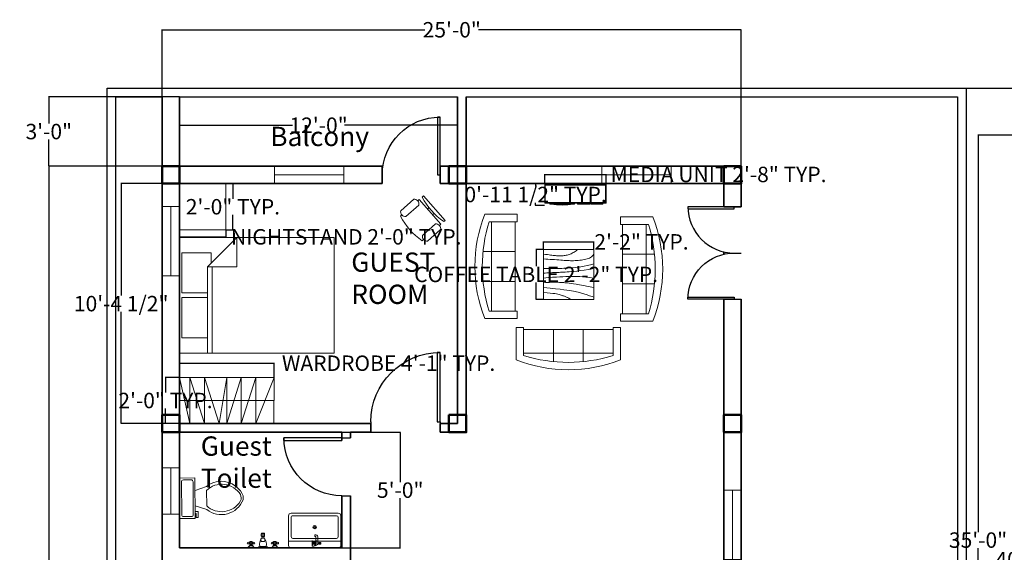
# Model space of a CAD drawing. Units: inches. Extents: x 20414 to 21627, y 49019 to 50314.
# Tile 2 of 10: x 20414 to 20925, y 49376 to 49652. Entities that reach past the tile are written whole.
import ezdxf

# ---------------------------------------------------------------- set-up
doc = ezdxf.new("R2010")
doc.units = ezdxf.units.IN
for name, color, linetype, lineweight in [('A-ANNO-DIMS', 7, 'Continuous', 18), ('A-AREA-IDEN', 7, 'Continuous', 18), ('A-FLOR-CASE', 2, 'Continuous', 18), ('A-FLOR-EDGE', 6, 'Continuous', 25), ('columns', 1, 'Continuous', 50), ('doors', 3, 'Continuous', 25), ('furniture', 2, 'Continuous', 18), ('plumbing', 1, 'Continuous', 18), ('walls', 6, 'Continuous', 35), ('windows', 3, 'Continuous', 18)]:
    doc.layers.add(name, color=color, linetype=linetype, lineweight=lineweight)
doc.styles.get("Standard").update_dxf_attribs({"font": 'arial.ttf'})
doc.dimstyles.get("Standard").update_dxf_attribs({"dimtxt": 8, "dimasz": 0.18, "dimexe": 0.18, "dimexo": 0.0625, "dimgap": 0.09, "dimtad": 0, "dimtih": 1, "dimtoh": 1, "dimdec": 1, "dimzin": 0, "dimdsep": 46, "dimlunit": 3, "dimtxsty": 'Standard', "dimcen": 0.09, "dimadec": 0, "dimazin": 0, "dimtfac": 1, "dimtdec": 1, "dimtofl": 0, "dimtmove": 0, "dimatfit": 3, "dimfxl": 1, "dimtolj": 1, "dimtzin": 0, "dimarcsym": 0})

# ---------------------------------------------------------------- blocks, each defined once
blk = doc.blocks.new('Bed - Queen')
for p, q in [((0, -80.00003), (0, 0)), ((0, 0), (59.99999, 0)), ((59.99999, 0), (59.99999, -80.00003)), ((7.99999, -1.2), (28.79998, -1.2)), ((7.99999, -14.4), (7.99999, -1.2)), ((28.79998, -1.2), (28.79998, -14.4)), ((31.19999, -1.2), (51.99999, -1.2)), ((31.19999, -14.4), (31.19999, -1.2)), ((51.99999, -1.2), (51.99999, -16.4)), ((0, -14.4), (44.8, -14.4)), ((59.99999, -29.6), (44.8, -14.4)), ((44.8, -14.4), (44.8, -29.6)), ((44.8, -16.8), (0, -16.8)), ((51.99999, -16.4), (46.79936, -16.4)), ((44.8, -29.6), (59.99999, -29.6)), ((59.99999, -80.00003), (0, -80.00003))]:
    blk.add_line(p, q)
blk = doc.blocks.new('Table - Square Woodgrain 42 x 42 in.')
blk.add_line((0, -42), (42, -42))
for points in [[(0, -4), (1.704, -4.2172), (3.2358, -4.4188), (4.615, -4.604), (5.8615, -4.7721), (6.9951, -4.9224), (8.0357, -5.0541), (9.0031, -5.1667), (9.9171, -5.2594), (10.7951, -5.3316), (11.6445, -5.3836), (12.4702, -5.4157), (13.277, -5.4283), (14.0698, -5.4217), (14.8535, -5.3964), (15.6331, -5.3526), (16.4133, -5.2908), (17.1986, -5.2103), (17.9913, -5.1062), (18.793, -4.9727), (19.6056, -4.8038), (20.4307, -4.5937), (21.2701, -4.3365), (22.1256, -4.0262), (22.9989, -3.6571), (23.888, -3.2272), (24.7756, -2.7516), (25.6408, -2.2491), (26.4624, -1.7387), (27.2195, -1.2395), (27.891, -0.7703), (28.456, -0.3501), (28.8934, 0.002)], [(0, -42), (0, 0), (42, 0), (42, -42)], [(0, -8), (1.8203, -8.1001), (3.6741, -8.2149), (5.5411, -8.3408), (7.4011, -8.4741), (9.2339, -8.6112), (11.0193, -8.7484), (12.7371, -8.8821), (14.3671, -9.0086), (15.8954, -9.1246), (17.3337, -9.2278), (18.6997, -9.3159), (20.0116, -9.387), (21.2871, -9.4389), (22.5442, -9.4696), (23.8008, -9.477), (25.0749, -9.459), (26.3791, -9.4137), (27.7049, -9.3403), (29.0383, -9.2382), (30.3655, -9.1068), (31.6728, -8.9455), (32.9461, -8.7535), (34.1717, -8.5304), (35.3358, -8.2756), (36.4268, -7.9863), (37.443, -7.6521), (38.3849, -7.2603), (39.253, -6.7986), (40.048, -6.2542), (40.7705, -5.6147), (41.421, -4.8674), (42, -4)], [(42, -12), (39.1784, -12.8621), (36.4519, -13.5654), (33.8246, -14.1294), (31.3004, -14.5731), (28.8832, -14.9161), (26.577, -15.1775), (24.3858, -15.3768), (22.3136, -15.5332), (20.3622, -15.6632), (18.5254, -15.7718), (16.7947, -15.8612), (15.1618, -15.9338), (13.6183, -15.9916), (12.1558, -16.0369), (10.7659, -16.0718), (9.4403, -16.0987), (8.1703, -16.1191), (6.9461, -16.1325), (5.7577, -16.1377), (4.595, -16.1335), (3.4479, -16.1188), (2.3064, -16.0924), (1.1604, -16.0532), (0, -16)], [(42, -16), (37.6529, -16.7365), (33.8802, -17.329), (30.6179, -17.7961), (27.8015, -18.1561), (25.3668, -18.4275), (23.2497, -18.6288), (21.3859, -18.7785), (19.7111, -18.8949), (18.1693, -18.9939), (16.7375, -19.0795), (15.401, -19.1534), (14.1449, -19.217), (12.9544, -19.2717), (11.8148, -19.3191), (10.7113, -19.3606), (9.6291, -19.3976), (8.5534, -19.4323), (7.47, -19.4689), (6.3643, -19.5122), (5.222, -19.5672), (4.0288, -19.6386), (2.7703, -19.7313), (1.4321, -19.8501), (0, -20)], [(0, -24), (3.9243, -23.6805), (7.4766, -23.4138), (10.6891, -23.1954), (13.5943, -23.0205), (16.2247, -22.8847), (18.6125, -22.7832), (20.7903, -22.7116), (22.7903, -22.6651), (24.6563, -22.642), (26.4764, -22.6507), (28.35, -22.7024), (30.3766, -22.8084), (32.6555, -22.98), (35.2861, -23.2283), (38.3678, -23.5645), (42, -24)], [(42, -32), (37.392, -31.017), (33.4585, -30.2231), (30.1291, -29.5949), (27.3334, -29.109), (25.0009, -28.742), (23.0612, -28.4707), (21.4439, -28.2716), (20.0786, -28.1215), (18.8998, -28.0002), (17.8609, -27.9014), (16.9206, -27.8219), (16.0371, -27.7588), (15.1691, -27.709), (14.2748, -27.6693), (13.3128, -27.6368), (12.2415, -27.6083), (11.0295, -27.5824), (9.6867, -27.5643), (8.233, -27.5608), (6.6884, -27.5787), (5.0728, -27.6248), (3.4062, -27.7058), (1.7086, -27.8286), (0, -28)], [(0, -32), (5.4026, -32.5358), (9.9494, -33.019), (13.7424, -33.4553), (16.8834, -33.8505), (19.4743, -34.2106), (21.6171, -34.5413), (23.4136, -34.8486), (24.9657, -35.1382), (26.3614, -35.4156), (27.6332, -35.6841), (28.7995, -35.9467), (29.8788, -36.2064), (30.8897, -36.4661), (31.8507, -36.7288), (32.7802, -36.9973), (33.6968, -37.2747), (34.6175, -37.5635), (35.5531, -37.8651), (36.5128, -38.1805), (37.506, -38.5108), (38.5421, -38.8568), (39.6302, -39.2197), (40.7797, -39.6004), (42, -40)], [(0, -36), (3.0098, -36.2857), (5.5354, -36.5643), (7.6368, -36.8359), (9.374, -37.1009), (10.807, -37.3597), (11.9957, -37.6126), (13.0002, -37.8599), (13.8804, -38.102), (14.6874, -38.3393), (15.4365, -38.5729), (16.1338, -38.8041), (16.7858, -39.0341), (17.3987, -39.264), (17.9787, -39.4952), (18.5322, -39.7288), (19.0655, -39.9662), (19.5832, -40.2081), (20.0842, -40.4544), (20.5657, -40.7046), (21.0249, -40.9581), (21.459, -41.2144), (21.8653, -41.4731), (22.2409, -41.7335), (22.5831, -41.9951)]]:
    blk.add_lwpolyline(points)
blk = doc.blocks.new('Toilet - top')
for p, q in [((9.5, -6), (9.5, -2)), ((-10, -8.5), (-8, -8.5)), ((-10, -9.5), (-10, -8.5)), ((-7, -9.5), (-10, -9.5)), ((-8, -8.5), (-8, -8)), ((-7, -8), (-7, -9.5)), ((-4, -8), (-6, -14)), ((4, -8), (6, -14)), ((4, -14), (-4, -14))]:
    blk.add_line(p, q)
blk.add_lwpolyline([(10.5, -8), (10.5, 0), (-10.5, 0), (-10.5, -8)], close=True)
for points in [[(-9.5, -2), (-9.5, -6)], [(8.5, -1), (-8.5, -1)], [(-8.5, -7), (8.5, -7)]]:
    blk.add_lwpolyline(points)
for centre, radius, start, end in [((-8.62, -1.88), 0.884, 81.8699, 188.1301), ((8.62, -1.88), 0.884, 351.8699, 98.1301), ((-8.62, -6.12), 0.884, 171.8699, 278.1301), ((8.62, -6.12), 0.884, 261.8699, 8.1301), ((3.52, -21.58), 12.17, 141.4691, 247.9714), ((4.2, -21.82), 11.33, 136.3677, 238.9468), ((-3.52, -21.58), 12.17, 292.0284, 38.5307), ((-4.2, -21.82), 11.33, 301.053, 43.6321), ((0, -27.88), 4, 245.7318, 294.2682), ((0, -29), 4, 254.8605, 285.1395)]:
    blk.add_arc(centre, radius, start, end)
blk = doc.blocks.new('Sofa - Roundback 7 ft.')
for p, q in [((-12.00002, -32.4421), (-12.00003, -6.5971)), ((11.99997, -32.4421), (11.99998, -6.5971)), ((-36.000027, -34), (-36.000027, -11.4696)), ((-35.999844, -13.3819), (35.9998, -13.3819)), ((35.99998, -34), (35.99998, -11.4696)), ((-36.000027, -32.4421), (35.99998, -32.4421))]:
    blk.add_line(p, q)
for points in [[(-36.000027, -34), (-42.000027, -34), (-42.000027, -8)], [(41.99998, -8), (41.99998, -34), (35.99998, -34)]]:
    blk.add_lwpolyline(points)
for centre, radius, start, end in [((0, -114.25), 114.25, 68.43141, 111.5686), ((-0.00001, -127.1968), 121.1968, 72.72033, 107.2797)]:
    blk.add_arc(centre, radius, start, end)
blk = doc.blocks.new('*U13')
for p, q in [((0, 0), (0, -6)), ((40, 0), (40, -6))]:
    blk.add_line(p, q)
blk.add_lwpolyline([(0, 0), (0, 40), (1.75, 40), (1.75, 0)], close=True)
blk.add_arc((0, 0), 40, 0, 90)
blk = doc.blocks.new('*U14')
for p, q in [((0, 0), (0, 6)), ((40, 0), (40, 6))]:
    blk.add_line(p, q)
blk.add_lwpolyline([(0, 0), (0, -40), (1.75, -40), (1.75, 0)], close=True)
blk.add_arc((0, 0), 40, 270, 0)
blk = doc.blocks.new('*U66')
for p, q in [((0, 0), (0, -6)), ((40, 0), (40, -6))]:
    blk.add_line(p, q)
blk.add_lwpolyline([(0, 0), (0, 40), (1.75, 40), (1.75, 0)], close=True)
blk.add_arc((0, 0), 40, 0, 90)
blk = doc.blocks.new('Entertainment Center')
for p, q in [((-4, 0), (-5, -1)), ((4, 0), (-4, 0)), ((5, -1), (4, 0)), ((-17, -19), (-17, -1)), ((-17, -1), (43, -1)), ((-16.5, -18.5), (-16.5, -1.5)), ((-16.5, -1.5), (42.5, -1.5)), ((42.5, -1.5), (42.5, -18.5)), ((43, -1), (43, -19)), ((43, -19), (-17, -19)), ((42.5, -18.5), (-16.5, -18.5)), ((-12, -20), (-12, -19)), ((12, -19), (12, -20)), ((15, -20), (15, -19)), ((27, -19), (27, -20)), ((28, -20), (28, -19)), ((40, -19), (40, -20)), ((12, -20), (-12, -20)), ((27, -20), (15, -20)), ((40, -20), (28, -20))]:
    blk.add_line(p, q)
blk.add_arc((0, 40), 61, 259.6111, 280.3889)
blk = doc.blocks.new('Faucet - Bathroom front')
for p, q in [((-0.5, 4.25), (0.5, 4.25)), ((0.5, 3.75), (-0.5, 3.75)), ((-0.5, 3), (0.5, 3)), ((-0.25, 3), (-0.25, 3.5)), ((0.25, 3.5), (0.25, 3)), ((-5, 0), (-2.25, 0)), ((-4.5087, 0.25), (-2.7408, 0.25)), ((-4, 1.625), (-4.25, 1.625)), ((-4, 1.375), (-4.25, 1.375)), ((-3.1442, 0.75), (-4.0979, 0.75)), ((-3.25, 1.625), (-3, 1.625)), ((-3.25, 1.375), (-3, 1.375)), ((-1.5, 0), (1.5, 0)), ((-1, 0.5), (1, 0.5)), ((0.5, 2), (-0.5, 2)), ((2.25, 0), (5, 0)), ((2.7413, 0.25), (4.5092, 0.25)), ((3.25, 1.625), (3, 1.625)), ((3.25, 1.375), (3, 1.375)), ((4.1058, 0.75), (3.1521, 0.75)), ((4, 1.625), (4.25, 1.625)), ((4, 1.375), (4.25, 1.375))]:
    blk.add_line(p, q)
for points in [[(-0.5, 3.75), (-0.5, 4.25)], [(-0.25, 4.5), (0.25, 4.5)], [(0.25, 3.5), (-0.25, 3.5)], [(0.5, 4.25), (0.5, 3.75)]]:
    blk.add_lwpolyline(points)
for points in [[(-4, 1), (-4, 2), (-3.25, 2), (-3.25, 1)], [(3.25, 1), (3.25, 2), (4, 2), (4, 1)]]:
    blk.add_lwpolyline(points, close=True)
for centre in [(-4.5, 1.5), (-3.625, 1.5), (-2.75, 1.5), (2.75, 1.5), (3.625, 1.5), (4.5, 1.5)]:
    blk.add_circle(centre, 0.2795)
for centre, radius, start, end in [((3, 1), 4.0311, 150.2551, 187.125), ((0.6413, 2.5), 1.246, 156.3417, 203.6583), ((-0.2575, 4.2575), 0.2426, 88.22243, 181.7776), ((-0.2575, 3.7425), 0.2426, 178.2224, 271.7776), ((0.2575, 4.2575), 0.2426, 358.2224, 91.77757), ((0.2575, 3.7425), 0.2426, 268.2224, 1.777565), ((-3, 1), 4.0311, 352.875, 29.74488), ((-0.6413, 2.5), 1.246, 336.3417, 23.65835), ((-5.375, 1.375), 1.4252, 285.2551, 344.7449), ((-1.875, 1.375), 1.4252, 195.2551, 254.7449), ((-0.7962, -0.2038), 0.7327, 106.1502, 163.8498), ((0.7962, -0.2038), 0.7327, 16.1502, 73.84979), ((1.875, 1.375), 1.4252, 285.2551, 344.7449), ((5.375, 1.375), 1.4252, 195.2551, 254.7449)]:
    blk.add_arc(centre, radius, start, end)
blk = doc.blocks.new('Sink-single - 30 in top')
blk.add_line((-15, -3.999996), (15, -3.999996))
for points in [[(-13.5, 0), (13.5, 0)], [(-15, -18.499996), (-15, -1.5)], [(-12.5, -5.499996), (12.5, -5.499996)], [(15, -1.5), (15, -18.499996)], [(-13.5, -17.499996), (-13.5, -6.499996)], [(13.5, -6.499996), (13.5, -17.499996)], [(13.5, -19.999996), (-13.5, -19.999996)], [(12.5, -18.499996), (-12.5, -18.499996)]]:
    blk.add_lwpolyline(points)
for radius in [1, 0.5]:
    blk.add_circle((0, -11.999996), radius)
for centre, radius, start, end in [((-13.5, -1.5), 1.5, 90, 180), ((-12.5, -6.499996), 1, 90, 180), ((12.5, -6.499996), 1, 0, 90), ((13.5, -1.5), 1.5, 0, 90), ((-13.5, -18.499996), 1.5, 180, 270), ((-12.5, -17.499996), 1, 180, 270), ((12.5, -17.499996), 1, 270, 0), ((13.5, -18.499996), 1.5, 270, 0)]:
    blk.add_arc(centre, radius, start, end)
blk = doc.blocks.new('Faucet - Bathroom side')
for p, q in [((-1.625, 0), (-1.375, 0)), ((-1.375, 0), (1.375, 0)), ((-0.88366, 0.25), (0.88424, 0.25)), ((-0.625, 4.25), (0.375, 4.25)), ((0.375, 3.75), (-0.625, 3.75)), ((-0.625, 3), (3.375, 3)), ((-0.375, 1.625), (-0.625, 1.625)), ((-0.375, 1.375), (-0.625, 1.375)), ((0.48078, 0.75), (-0.47286, 0.75)), ((-0.375, 3), (-0.375, 3.5)), ((0.125, 3.5), (0.125, 3)), ((2.875, 2), (0.375, 2)), ((0.375, 1.625), (0.625, 1.625)), ((0.375, 1.375), (0.625, 1.375)), ((4.375, 1.5), (3.375, 1.5))]:
    blk.add_line(p, q)
for points in [[(-0.625, 3.75), (-0.625, 4.25)], [(-0.375, 4.5), (0.125, 4.5)], [(0.125, 3.5), (-0.375, 3.5)], [(0.375, 4.25), (0.375, 3.75)]]:
    blk.add_lwpolyline(points)
blk.add_lwpolyline([(-0.375, 1), (-0.375, 2), (0.375, 2), (0.375, 1)], close=True)
for centre in [(-0.875, 1.5), (0, 1.5), (0.875, 1.5)]:
    blk.add_circle(centre, 0.27951)
for centre, radius, start, end in [((3.45929, -0.0281), 5.08436, 143.4467, 179.6834), ((-1.75, 1.375), 1.42522, 285.2551, 344.7449), ((-0.38253, 4.2575), 0.24259, 88.22243, 181.7776), ((-0.38253, 3.7424), 0.24259, 178.2224, 271.7776), ((0.13252, 4.2575), 0.24259, 358.2224, 91.77757), ((0.13252, 3.7424), 0.24259, 268.2224, 1.777565), ((1.75, 1.375), 1.42522, 195.2551, 254.7449), ((-2.49562, -0.286), 3.38273, 9.709485, 29.48735), ((2.96867, 1.5936), 0.41699, 347.0192, 102.9808), ((2.70708, 1.4714), 1.66816, 0.9827695, 66.39737)]:
    blk.add_arc(centre, radius, start, end)
blk = doc.blocks.new('Chair - Desk')
for p, q in [((-8.5, 0), (-8.5, -1)), ((-8.5, 0), (8.5, 0)), ((8.5, 0), (8.5, -1)), ((-10.5, -5), (-10.5, -14)), ((-8.5, -3), (-8.5, -4)), ((-8.5, -3), (8.5, -3)), ((-6.5, -14), (-6.5, -5)), ((-2, -3), (-2, -1.9355)), ((2, -1.9576), (2, -3)), ((6.5, -5), (6.5, -14)), ((8.5, -3), (8.5, -4)), ((10.5, -14), (10.5, -5)), ((-8.5, -15), (-8.5, -16)), ((8.5, -15), (8.5, -16))]:
    blk.add_line(p, q)
for centre, radius, start, end in [((-8.5, -6.5), 2.5, 36.8699, 143.1301), ((0, 34.625), 36.625, 256.5803, 283.4197), ((8.5, -6.5), 2.5, 36.8699, 143.1301), ((-8.5, -12.5), 2.5, 216.8699, 323.1301), ((8.5, -12.5), 2.5, 216.8699, 323.1301), ((0, 19.625), 36.625, 256.5803, 283.4197)]:
    blk.add_arc(centre, radius, start, end)
blk = doc.blocks.new('*U28')
for p, q in [((-40, 0), (-40, 6)), ((0, 0), (0, 6))]:
    blk.add_line(p, q)
blk.add_lwpolyline([(0, 0), (0, -40), (-1.75, -40), (-1.75, 0)], close=True)
blk.add_arc((0, 0), 40, 180, 270)
blk = doc.blocks.new('WINDOW-36IN-PLAN')
for p, q in [((9, 36), (0, 36)), ((4.5, 36), (4.5, 0)), ((9, 0), (0, 0))]:
    blk.add_line(p, q)
blk = doc.blocks.new('VENT-24IN-PLAN')
for p, q in [((9, 24), (0, 24)), ((4.5, 0), (4.5, 24)), ((9, 0), (0, 0))]:
    blk.add_line(p, q)
blk = doc.blocks.new('COLUMN-9X9')
blk.add_lwpolyline([(0, 9), (0, 0), (9, 0), (9, 9), (0, 9)])
blk = doc.blocks.new('NIGHTSTAND-24IN')
blk.add_lwpolyline([(0, 0), (0, 24), (24, 24), (24, 0), (0, 0)])
blk = doc.blocks.new('WARDROBE-49IN')
for q in [(0, 24), (48.87, 0)]:
    blk.add_line((49, 24), q)
blk.add_lwpolyline([(0, 24), (5.3, 0), (5.3, 24), (12.93, 0), (12.93, 24), (20.56, 0), (24.5, 24), (24.5, 0), (31.88, 24), (31.88, 0), (39.51, 24), (39.51, 0), (49, 24), (48.94, 12), (0, 12)])
blk = doc.blocks.new('*D88')
at = {"layer": 'A-ANNO-DIMS', "color": 0, "lineweight": -2, "transparency": 16777216}
for p, q in [((20497.19, 49543.2), (20497.19, 49539.49)), ((20521.19, 49543.2), (20521.19, 49539.49)), ((20497.37, 49539.67), (20521.01, 49539.67)), ((20521.19, 49539.67), (20521.37, 49539.67))]:
    blk.add_line(p, q, dxfattribs=at)
at = {"layer": 'A-ANNO-DIMS', "color": 0, "transparency": 16777216}
for points in [[(20497.37, 49539.7), (20497.37, 49539.64), (20497.19, 49539.67)], [(20521.01, 49539.7), (20521.01, 49539.64), (20521.19, 49539.67)]]:
    blk.add_solid(points, dxfattribs=at)
at = {"layer": 'Defpoints', "color": 0, "transparency": 16777216}
for p in [(20497.19, 49543.27), (20521.19, 49543.27), (20521.19, 49539.67)]:
    blk.add_point(p, dxfattribs=at)
at = {"layer": 'A-ANNO-DIMS', "color": 0, "transparency": 16777216, "insert": (20583.52, 49539.67), "char_height": 8, "attachment_point": 5}
blk.add_mtext('\\A1;NIGHTSTAND 2\'-0" TYP.', dxfattribs=at)
blk = doc.blocks.new('*D89')
at = {"layer": 'A-ANNO-DIMS', "color": 0, "lineweight": -2, "transparency": 16777216}
for p, q in [((20521.25, 49567.27), (20524.97, 49567.27)), ((20524.79, 49567.09), (20524.79, 49559.44)), ((20524.79, 49543.45), (20524.79, 49551.09)), ((20521.25, 49543.27), (20524.97, 49543.27))]:
    blk.add_line(p, q, dxfattribs=at)
at = {"layer": 'A-ANNO-DIMS', "color": 0, "transparency": 16777216}
for points in [[(20524.76, 49567.09), (20524.82, 49567.09), (20524.79, 49567.27)], [(20524.76, 49543.45), (20524.82, 49543.45), (20524.79, 49543.27)]]:
    blk.add_solid(points, dxfattribs=at)
at = {"layer": 'Defpoints', "color": 0, "transparency": 16777216}
for p in [(20521.19, 49567.27), (20524.79, 49567.27), (20521.19, 49543.27)]:
    blk.add_point(p, dxfattribs=at)
at = {"layer": 'A-ANNO-DIMS', "color": 0, "transparency": 16777216, "insert": (20524.79, 49555.27), "char_height": 8, "attachment_point": 5}
blk.add_mtext('\\A1;2\'-0" TYP.', dxfattribs=at)
blk = doc.blocks.new('*D102')
at = {"layer": 'A-ANNO-DIMS', "color": 0, "lineweight": -2, "transparency": 16777216}
for p, q in [((20685.72, 49533.16), (20681.7, 49533.16)), ((20681.88, 49532.98), (20681.88, 49524.39)), ((20681.88, 49507.34), (20681.88, 49515.93)), ((20685.72, 49507.16), (20681.7, 49507.16))]:
    blk.add_line(p, q, dxfattribs=at)
at = {"layer": 'A-ANNO-DIMS', "color": 0, "transparency": 16777216}
for points in [[(20681.85, 49532.98), (20681.91, 49532.98), (20681.88, 49533.16)], [(20681.85, 49507.34), (20681.91, 49507.34), (20681.88, 49507.16)]]:
    blk.add_solid(points, dxfattribs=at)
at = {"layer": 'Defpoints', "color": 0, "transparency": 16777216}
for p in [(20681.88, 49533.16), (20685.78, 49533.16), (20685.78, 49507.16)]:
    blk.add_point(p, dxfattribs=at)
at = {"layer": 'A-ANNO-DIMS', "color": 0, "transparency": 16777216, "insert": (20681.88, 49520.16), "char_height": 8, "attachment_point": 5}
blk.add_mtext('\\A1;COFFEE TABLE 2\'-2" TYP.', dxfattribs=at)
blk = doc.blocks.new('*D103')
at = {"layer": 'A-ANNO-DIMS', "color": 0, "lineweight": -2, "transparency": 16777216}
for p, q in [((20685.78, 49533.22), (20685.78, 49537.24)), ((20685.96, 49537.06), (20711.6, 49537.06)), ((20711.78, 49533.22), (20711.78, 49537.24)), ((20711.78, 49537.06), (20711.96, 49537.06))]:
    blk.add_line(p, q, dxfattribs=at)
at = {"layer": 'A-ANNO-DIMS', "color": 0, "transparency": 16777216}
for points in [[(20685.96, 49537.09), (20685.96, 49537.03), (20685.78, 49537.06)], [(20711.6, 49537.09), (20711.6, 49537.03), (20711.78, 49537.06)]]:
    blk.add_solid(points, dxfattribs=at)
at = {"layer": 'Defpoints', "color": 0, "transparency": 16777216}
for p in [(20711.78, 49537.06), (20685.78, 49533.16), (20711.78, 49533.16)]:
    blk.add_point(p, dxfattribs=at)
at = {"layer": 'A-ANNO-DIMS', "color": 0, "transparency": 16777216, "insert": (20736.5, 49537.06), "char_height": 8, "attachment_point": 5}
blk.add_mtext('\\A1;2\'-2" TYP.', dxfattribs=at)
blk = doc.blocks.new('*D104')
at = {"layer": 'A-ANNO-DIMS', "color": 0, "lineweight": -2, "transparency": 16777216}
for p, q in [((20686.38, 49567.33), (20686.38, 49572.21)), ((20686.56, 49572.03), (20717.97, 49572.03)), ((20718.15, 49567.33), (20718.15, 49572.21)), ((20718.15, 49572.03), (20718.33, 49572.03))]:
    blk.add_line(p, q, dxfattribs=at)
at = {"layer": 'A-ANNO-DIMS', "color": 0, "transparency": 16777216}
for points in [[(20686.56, 49572.06), (20686.56, 49572), (20686.38, 49572.03)], [(20717.97, 49572.06), (20717.97, 49572), (20718.15, 49572.03)]]:
    blk.add_solid(points, dxfattribs=at)
at = {"layer": 'Defpoints', "color": 0, "transparency": 16777216}
for p in [(20718.15, 49572.03), (20686.38, 49567.27), (20718.15, 49567.27)]:
    blk.add_point(p, dxfattribs=at)
at = {"layer": 'A-ANNO-DIMS', "color": 0, "transparency": 16777216, "insert": (20776.45, 49572.03), "char_height": 8, "attachment_point": 5}
blk.add_mtext('\\A1;MEDIA UNIT 2\'-8" TYP.', dxfattribs=at)
blk = doc.blocks.new('*D105')
at = {"layer": 'A-ANNO-DIMS', "color": 0, "lineweight": -2, "transparency": 16777216}
for p, q in [((20686.32, 49567.27), (20681.44, 49567.27)), ((20681.62, 49567.09), (20681.62, 49565.84)), ((20681.62, 49556.15), (20681.62, 49557.39)), ((20686.32, 49555.97), (20681.44, 49555.97))]:
    blk.add_line(p, q, dxfattribs=at)
at = {"layer": 'A-ANNO-DIMS', "color": 0, "transparency": 16777216}
for points in [[(20681.59, 49567.09), (20681.65, 49567.09), (20681.62, 49567.27)], [(20681.59, 49556.15), (20681.65, 49556.15), (20681.62, 49555.97)]]:
    blk.add_solid(points, dxfattribs=at)
at = {"layer": 'Defpoints', "color": 0, "transparency": 16777216}
for p in [(20681.62, 49567.27), (20686.38, 49567.27), (20686.38, 49555.97)]:
    blk.add_point(p, dxfattribs=at)
at = {"layer": 'A-ANNO-DIMS', "color": 0, "transparency": 16777216, "insert": (20681.62, 49561.62), "char_height": 8, "attachment_point": 5}
blk.add_mtext('\\A1;0\'-11 1/2" TYP.', dxfattribs=at)
blk = doc.blocks.new('*D108')
at = {"layer": 'A-ANNO-DIMS', "color": 0, "lineweight": -2, "transparency": 16777216}
for p, q in [((20497.18, 49466.83), (20497.18, 49474.3)), ((20497.36, 49474.12), (20546, 49474.12)), ((20546.18, 49466.83), (20546.18, 49474.3)), ((20546.18, 49474.12), (20546.36, 49474.12))]:
    blk.add_line(p, q, dxfattribs=at)
at = {"layer": 'A-ANNO-DIMS', "color": 0, "transparency": 16777216}
for points in [[(20497.36, 49474.15), (20497.36, 49474.09), (20497.18, 49474.12)], [(20546, 49474.15), (20546, 49474.09), (20546.18, 49474.12)]]:
    blk.add_solid(points, dxfattribs=at)
at = {"layer": 'Defpoints', "color": 0, "transparency": 16777216}
for p in [(20546.18, 49474.12), (20497.18, 49466.77), (20546.18, 49466.77)]:
    blk.add_point(p, dxfattribs=at)
at = {"layer": 'A-ANNO-DIMS', "color": 0, "transparency": 16777216, "insert": (20605.45, 49474.12), "char_height": 8, "attachment_point": 5}
blk.add_mtext('\\A1;WARDROBE 4\'-1" TYP.', dxfattribs=at)
blk = doc.blocks.new('*D109')
at = {"layer": 'A-ANNO-DIMS', "color": 0, "lineweight": -2, "transparency": 16777216}
for p, q in [((20497.11, 49466.77), (20489.65, 49466.77)), ((20489.83, 49466.59), (20489.83, 49458.94)), ((20489.83, 49442.95), (20489.83, 49450.59)), ((20497.11, 49442.77), (20489.65, 49442.77))]:
    blk.add_line(p, q, dxfattribs=at)
at = {"layer": 'A-ANNO-DIMS', "color": 0, "transparency": 16777216}
for points in [[(20489.8, 49466.59), (20489.86, 49466.59), (20489.83, 49466.77)], [(20489.8, 49442.95), (20489.86, 49442.95), (20489.83, 49442.77)]]:
    blk.add_solid(points, dxfattribs=at)
at = {"layer": 'Defpoints', "color": 0, "transparency": 16777216}
for p in [(20489.83, 49466.77), (20497.18, 49466.77), (20497.18, 49442.77)]:
    blk.add_point(p, dxfattribs=at)
at = {"layer": 'A-ANNO-DIMS', "color": 0, "transparency": 16777216, "insert": (20489.83, 49454.77), "char_height": 8, "attachment_point": 5}
blk.add_mtext('\\A1;2\'-0" TYP.', dxfattribs=at)
blk = doc.blocks.new('*D121')
at = {"layer": 'A-ANNO-DIMS', "color": 0, "lineweight": -2, "transparency": 16777216}
for p, q in [((20904.74, 49616.77), (20935.16, 49616.77)), ((20934.98, 49616.59), (20934.98, 49376.44)), ((20934.98, 49127.95), (20934.98, 49368.09)), ((20904.74, 49127.77), (20935.16, 49127.77))]:
    blk.add_line(p, q, dxfattribs=at)
at = {"layer": 'A-ANNO-DIMS', "color": 0, "transparency": 16777216}
for points in [[(20934.95, 49616.59), (20935.01, 49616.59), (20934.98, 49616.77)], [(20934.95, 49127.95), (20935.01, 49127.95), (20934.98, 49127.77)]]:
    blk.add_solid(points, dxfattribs=at)
at = {"layer": 'Defpoints', "color": 0, "transparency": 16777216}
for p in [(20904.68, 49616.77), (20934.98, 49616.77), (20904.68, 49127.77)]:
    blk.add_point(p, dxfattribs=at)
at = {"layer": 'A-ANNO-DIMS', "color": 0, "transparency": 16777216, "insert": (20934.98, 49372.27), "char_height": 8, "attachment_point": 5}
blk.add_mtext('\\A1;40\'-9"', dxfattribs=at)
blk = doc.blocks.new('*D122')
at = {"layer": 'A-ANNO-DIMS', "color": 0, "lineweight": -2, "transparency": 16777216}
for p, q in [((20488.18, 49576.33), (20488.18, 49647.25)), ((20488.36, 49647.07), (20624.28, 49647.07)), ((20788, 49647.07), (20652.08, 49647.07)), ((20788.18, 49576.33), (20788.18, 49647.25))]:
    blk.add_line(p, q, dxfattribs=at)
at = {"layer": 'A-ANNO-DIMS', "color": 0, "transparency": 16777216}
for points in [[(20488.36, 49647.1), (20488.36, 49647.04), (20488.18, 49647.07)], [(20788, 49647.1), (20788, 49647.04), (20788.18, 49647.07)]]:
    blk.add_solid(points, dxfattribs=at)
at = {"layer": 'Defpoints', "color": 0, "transparency": 16777216}
for p in [(20788.18, 49647.07), (20488.18, 49576.27), (20788.18, 49576.27)]:
    blk.add_point(p, dxfattribs=at)
at = {"layer": 'A-ANNO-DIMS', "color": 0, "transparency": 16777216, "insert": (20638.18, 49647.07), "char_height": 8, "attachment_point": 5}
blk.add_mtext('\\A1;25\'-0"', dxfattribs=at)
blk = doc.blocks.new('*D123')
at = {"layer": 'A-ANNO-DIMS', "color": 0, "lineweight": -2, "transparency": 16777216}
for p, q in [((20488.11, 49576.27), (20429.2, 49576.27)), ((20429.38, 49576.09), (20429.38, 49370.44)), ((20429.38, 49156.45), (20429.38, 49362.09)), ((20488.11, 49156.27), (20429.2, 49156.27))]:
    blk.add_line(p, q, dxfattribs=at)
at = {"layer": 'A-ANNO-DIMS', "color": 0, "transparency": 16777216}
for points in [[(20429.35, 49576.09), (20429.41, 49576.09), (20429.38, 49576.27)], [(20429.35, 49156.45), (20429.41, 49156.45), (20429.38, 49156.27)]]:
    blk.add_solid(points, dxfattribs=at)
at = {"layer": 'Defpoints', "color": 0, "transparency": 16777216}
for p in [(20429.38, 49576.27), (20488.18, 49576.27), (20488.18, 49156.27)]:
    blk.add_point(p, dxfattribs=at)
at = {"layer": 'A-ANNO-DIMS', "color": 0, "transparency": 16777216, "insert": (20429.38, 49366.27), "char_height": 8, "attachment_point": 5}
blk.add_mtext('\\A1;35\'-0"', dxfattribs=at)
blk = doc.blocks.new('*D126')
at = {"layer": 'A-ANNO-DIMS', "color": 0, "lineweight": -2, "transparency": 16777216}
for p, q in [((20497.11, 49612.27), (20429.2, 49612.27)), ((20429.38, 49612.09), (20429.38, 49598.44)), ((20429.38, 49576.45), (20429.38, 49590.09)), ((20497.13, 49576.27), (20429.2, 49576.27))]:
    blk.add_line(p, q, dxfattribs=at)
at = {"layer": 'A-ANNO-DIMS', "color": 0, "transparency": 16777216}
for points in [[(20429.35, 49612.09), (20429.41, 49612.09), (20429.38, 49612.27)], [(20429.35, 49576.45), (20429.41, 49576.45), (20429.38, 49576.27)]]:
    blk.add_solid(points, dxfattribs=at)
at = {"layer": 'Defpoints', "color": 0, "transparency": 16777216}
for p in [(20429.38, 49612.27), (20497.18, 49612.27), (20497.19, 49576.27)]:
    blk.add_point(p, dxfattribs=at)
at = {"layer": 'A-ANNO-DIMS', "color": 0, "transparency": 16777216, "insert": (20429.38, 49594.27), "char_height": 8, "attachment_point": 5}
blk.add_mtext('\\A1;3\'-0"', dxfattribs=at)
blk = doc.blocks.new('*D127')
at = {"layer": 'A-ANNO-DIMS', "color": 0, "lineweight": -2, "transparency": 16777216}
for p, q in [((20497.11, 49567.27), (20466.7, 49567.27)), ((20466.88, 49567.09), (20466.88, 49509.24)), ((20466.88, 49442.95), (20466.88, 49500.79)), ((20497.11, 49442.77), (20466.7, 49442.77))]:
    blk.add_line(p, q, dxfattribs=at)
at = {"layer": 'A-ANNO-DIMS', "color": 0, "transparency": 16777216}
for points in [[(20466.85, 49567.09), (20466.91, 49567.09), (20466.88, 49567.27)], [(20466.85, 49442.95), (20466.91, 49442.95), (20466.88, 49442.77)]]:
    blk.add_solid(points, dxfattribs=at)
at = {"layer": 'Defpoints', "color": 0, "transparency": 16777216}
for p in [(20466.88, 49567.27), (20497.18, 49567.27), (20497.18, 49442.77)]:
    blk.add_point(p, dxfattribs=at)
at = {"layer": 'A-ANNO-DIMS', "color": 0, "transparency": 16777216, "insert": (20466.88, 49505.02), "char_height": 8, "attachment_point": 5}
blk.add_mtext('\\A1;10\'-4 1/2"', dxfattribs=at)
blk = doc.blocks.new('*D129')
at = {"layer": 'A-ANNO-DIMS', "color": 0, "lineweight": -2, "transparency": 16777216}
for p, q in [((20497.18, 49567.33), (20497.18, 49597.75)), ((20497.36, 49597.57), (20555.72, 49597.57)), ((20641, 49597.57), (20582.63, 49597.57)), ((20641.18, 49567.33), (20641.18, 49597.75))]:
    blk.add_line(p, q, dxfattribs=at)
at = {"layer": 'A-ANNO-DIMS', "color": 0, "transparency": 16777216}
for points in [[(20497.36, 49597.6), (20497.36, 49597.54), (20497.18, 49597.57)], [(20641, 49597.6), (20641, 49597.54), (20641.18, 49597.57)]]:
    blk.add_solid(points, dxfattribs=at)
at = {"layer": 'Defpoints', "color": 0, "transparency": 16777216}
for p in [(20641.18, 49597.57), (20497.18, 49567.27), (20641.18, 49567.27)]:
    blk.add_point(p, dxfattribs=at)
at = {"layer": 'A-ANNO-DIMS', "color": 0, "transparency": 16777216, "insert": (20569.18, 49597.57), "char_height": 8, "attachment_point": 5}
blk.add_mtext('\\A1;12\'-0"', dxfattribs=at)
blk = doc.blocks.new('*D131')
at = {"layer": 'A-ANNO-DIMS', "color": 0, "lineweight": -2, "transparency": 16777216}
for p, q in [((20581.24, 49438.27), (20611.66, 49438.27)), ((20611.48, 49438.09), (20611.48, 49412.44)), ((20611.48, 49378.45), (20611.48, 49404.09)), ((20581.24, 49378.27), (20611.66, 49378.27))]:
    blk.add_line(p, q, dxfattribs=at)
at = {"layer": 'A-ANNO-DIMS', "color": 0, "transparency": 16777216}
for points in [[(20611.45, 49438.09), (20611.51, 49438.09), (20611.48, 49438.27)], [(20611.45, 49378.45), (20611.51, 49378.45), (20611.48, 49378.27)]]:
    blk.add_solid(points, dxfattribs=at)
at = {"layer": 'Defpoints', "color": 0, "transparency": 16777216}
for p in [(20581.18, 49438.27), (20581.18, 49378.27), (20611.48, 49378.27)]:
    blk.add_point(p, dxfattribs=at)
at = {"layer": 'A-ANNO-DIMS', "color": 0, "transparency": 16777216, "insert": (20611.48, 49408.27), "char_height": 8, "attachment_point": 5}
blk.add_mtext('\\A1;5\'-0"', dxfattribs=at)
blk = doc.blocks.new('*D136')
at = {"layer": 'A-ANNO-DIMS', "color": 0, "lineweight": -2, "transparency": 16777216}
for p, q in [((20969.98, 49592.35), (20910.71, 49592.35)), ((20910.89, 49592.17), (20910.89, 49386.52)), ((20910.89, 49172.53), (20910.89, 49378.17)), ((20969.98, 49172.35), (20910.71, 49172.35))]:
    blk.add_line(p, q, dxfattribs=at)
at = {"layer": 'A-ANNO-DIMS', "color": 0, "transparency": 16777216}
for points in [[(20910.86, 49592.17), (20910.92, 49592.17), (20910.89, 49592.35)], [(20910.86, 49172.53), (20910.92, 49172.53), (20910.89, 49172.35)]]:
    blk.add_solid(points, dxfattribs=at)
at = {"layer": 'Defpoints', "color": 0, "transparency": 16777216}
for p in [(20910.89, 49592.35), (20970.04, 49592.35), (20970.04, 49172.35)]:
    blk.add_point(p, dxfattribs=at)
at = {"layer": 'A-ANNO-DIMS', "color": 0, "transparency": 16777216, "insert": (20910.89, 49382.35), "char_height": 8, "attachment_point": 5}
blk.add_mtext('\\A1;35\'-0"', dxfattribs=at)

msp = doc.modelspace()

# ---------------------------------------------------------------- linework, layer by layer
at = {"layer": 'A-FLOR-EDGE'}
for p, q in [((20488.19, 49616.77), (20904.68, 49616.77)), ((20904.68, 49616.77), (20904.68, 49156.27)), ((20497.18, 49612.27), (20641.18, 49612.27)), ((20645.68, 49612.27), (20864.18, 49612.27)), ((20864.18, 49612.27), (20900.18, 49612.27)), ((20900.18, 49612.27), (20900.18, 49156.27))]:
    msp.add_line(p, q, dxfattribs=at)
for points in [[(20904.68, 49156.27), (20904.68, 49127.77), (20488.18, 49127.77), (20459.68, 49127.77), (20459.68, 49616.77), (20488.19, 49616.77)], [(20900.18, 49156.27), (20900.18, 49132.27), (20488.18, 49132.27), (20464.18, 49132.27), (20464.18, 49612.27), (20488.19, 49612.27)]]:
    msp.add_lwpolyline(points, dxfattribs=at)
at = {"layer": 'doors'}
for p, q in [((20779.18, 49555.27), (20788.18, 49555.27)), ((20788.18, 49555.27), (20779.18, 49555.27)), ((20779.18, 49507.27), (20788.18, 49507.27)), ((20779.18, 49507.27), (20788.18, 49507.27))]:
    msp.add_line(p, q, dxfattribs=at)
at = {"layer": 'walls'}
for p, q in [((20488.18, 49156.27), (20488.18, 49612.27)), ((20497.18, 49442.77), (20497.18, 49612.27)), ((20641.18, 49442.77), (20641.18, 49612.27)), ((20645.68, 49438.27), (20645.68, 49612.27)), ((20488.18, 49576.27), (20602.18, 49576.27)), ((20602.18, 49567.27), (20602.18, 49576.27)), ((20632.18, 49567.27), (20632.18, 49576.27)), ((20632.18, 49576.27), (20788.18, 49576.27)), ((20788.18, 49576.27), (20788.18, 49555.27)), ((20497.18, 49567.27), (20602.18, 49567.27)), ((20632.18, 49567.27), (20641.18, 49567.27)), ((20645.68, 49567.27), (20779.18, 49567.27)), ((20779.18, 49567.27), (20779.18, 49555.27)), ((20779.18, 49531.88), (20779.18, 49530.65)), ((20779.18, 49507.27), (20779.18, 49442.77)), ((20788.18, 49507.27), (20788.18, 49156.27)), ((20546.05, 49442.77), (20497.18, 49442.77)), ((20596.18, 49442.77), (20546.05, 49442.77)), ((20596.18, 49438.27), (20596.18, 49442.77)), ((20641.18, 49442.77), (20632.18, 49442.77)), ((20632.18, 49438.27), (20632.18, 49442.77)), ((20546.05, 49438.27), (20497.18, 49438.27)), ((20497.18, 49378.27), (20497.18, 49438.27)), ((20581.18, 49438.27), (20546.05, 49438.27)), ((20581.18, 49434.05), (20581.18, 49438.27)), ((20596.18, 49438.27), (20585.68, 49438.27)), ((20585.68, 49435.36), (20585.68, 49438.27)), ((20645.68, 49438.27), (20632.18, 49438.27)), ((20779.18, 49438.27), (20779.18, 49402.27)), ((20581.18, 49378.27), (20581.18, 49405.36)), ((20585.68, 49313.77), (20585.68, 49405.36)), ((20585.68, 49378.27), (20585.68, 49405.36)), ((20779.18, 49407.94), (20779.18, 49313.77)), ((20581.18, 49378.27), (20497.18, 49378.27))]:
    msp.add_line(p, q, dxfattribs=at)

# ---------------------------------------------------------------- block references
at = {"layer": 'A-FLOR-CASE'}
msp.add_blockref('WARDROBE-49IN', (20497.18, 49442.77), dxfattribs=at)
at = {"layer": 'columns'}
for p in [(20488.19, 49567.27), (20636.68, 49567.27), (20779.18, 49567.27), (20488.18, 49438.27), (20636.68, 49438.27), (20779.18, 49438.27)]:
    msp.add_blockref('COLUMN-9X9', p, dxfattribs=at)
at = {"layer": 'doors'}
for name, p, xscale, yscale, zscale, rotation in [('*U28', (20632.18, 49571.77), -0.75, 0.75, 0.75, 180), ('*U14', (20784.58, 49555.27), 0.6, 0.6, 0.6, 270), ('*U14', (20784.58, 49507.27), -0.6, 0.6, 0.6, 270), ('*U66', (20581.18, 49435.36), -0.75, 0.75, 0.75, 90.00000000009263)]:
    msp.add_blockref(name, p, dxfattribs=dict(at, xscale=xscale, yscale=yscale, zscale=zscale, rotation=rotation))
at = {"layer": 'doors', "xscale": -0.9, "yscale": 0.9, "zscale": 0.9}
msp.add_blockref('*U13', (20632.18, 49443.67), dxfattribs=at)
at = {"layer": 'furniture'}
msp.add_blockref('NIGHTSTAND-24IN', (20497.19, 49543.27), dxfattribs=at)
for name, p, rotation in [('Chair - Desk', (20629.19, 49554.58), 311.4332562192998), ('Bed - Queen', (20497.18, 49479.36), 90)]:
    msp.add_blockref(name, p, dxfattribs=dict(at, rotation=rotation))
for name, p, xscale, yscale, zscale in [('Entertainment Center', (20695.38, 49567.27), 0.5294023735262411, 0.5294023735262411, 0.5294023735262411), ('Table - Square Woodgrain 42 x 42 in.', (20685.78, 49533.16), 0.6190476190476191, 0.6190476190476191, 0.6190476190476191)]:
    msp.add_blockref(name, p, dxfattribs=dict(at, xscale=xscale, yscale=yscale, zscale=zscale))
at = {"layer": 'furniture', "yscale": 0.6442431863649634, "zscale": 0.6442431863649634}
for p, xscale, rotation in [((20650.15, 49524.31), 0.6442431863649634, 90), ((20747.49, 49522.95), -0.6442431863649634, 270), ((20698.6, 49470.7), -0.6442431863649634, 180)]:
    msp.add_blockref('Sofa - Roundback 7 ft.', p, dxfattribs=dict(at, xscale=xscale, rotation=rotation))
at = {"layer": 'plumbing', "rotation": 90.45084889114678}
msp.add_blockref('Toilet - top', (20497.18, 49404.05), dxfattribs=at)
at = {"layer": 'plumbing', "xscale": 0.9035913028591334, "yscale": 0.9035913028591334, "zscale": 0.9035913028591334, "rotation": 180}
msp.add_blockref('Sink-single - 30 in top', (20567.16, 49378.27), dxfattribs=at)
at = {"layer": 'plumbing', "xscale": 1.701154593653001, "yscale": 1.701154593653001, "zscale": 1.701154593653001}
msp.add_blockref('Faucet - Bathroom front', (20540.36, 49378.27), dxfattribs=at)
at = {"layer": 'plumbing', "xscale": -1, "rotation": 270.803393295101}
msp.add_blockref('Faucet - Bathroom side', (20565.85, 49380.76), dxfattribs=at)
at = {"layer": 'windows'}
for p, rotation in [((20546.32, 49576.27), 269.9999999999809), ((20715.91, 49576.27), 270.0000000000218), ((20497.18, 49555.39), 180), ((20788.18, 49408.29), 180)]:
    msp.add_blockref('WINDOW-36IN-PLAN', p, dxfattribs=dict(at, rotation=rotation))
msp.add_blockref('VENT-24IN-PLAN', (20488.18, 49395.87), dxfattribs=at)

# ---------------------------------------------------------------- texts
at = {"layer": 'A-AREA-IDEN', "char_height": 10, "attachment_point": 1}
for s, width, heights, insert in [('Balcony', 44.4717, [34.97], (20544.13, 49596.74)), ('GUEST\\PROOM', 44.4717, [34.97], (20586.11, 49531.52)), ('Guest\\PToilet', 43.1663, [28.71], (20508.14, 49436.14))]:
    msp.add_mtext_dynamic_manual_height_columns(s, width=width, gutter_width=50, heights=heights, dxfattribs=dict(at, insert=insert))

# ---------------------------------------------------------------- dimensions: what is measured, and where the dimension line sits
at = {"layer": 'A-ANNO-DIMS'}
for base, p1, p2, picture, middle in [((20788.18, 49647.07), (20488.18, 49576.27), (20788.18, 49576.27), '*D122', (20638.18, 49647.07)), ((20641.18, 49597.57), (20497.18, 49567.27), (20641.18, 49567.27), '*D129', (20569.18, 49597.57))]:
    dim = msp.add_linear_dim(base=base, p1=p1, p2=p2, dimstyle='Standard', override={"dimdec": 1, "dimlfac": 1, "dimrnd": 0, "dimzin": 1, "dimdsep": 46, "dimlunit": 4, "dimfrac": 2}, dxfattribs=at)
    dim.commit()
    dim.dimension.update_dxf_attribs({"geometry": picture, "text_midpoint": middle})
for base, p1, p2, angle, picture, middle in [((20934.98, 49616.77), (20904.68, 49127.77), (20904.68, 49616.77), 90, '*D121', (20934.98, 49372.27)), ((20429.38, 49612.27), (20497.19, 49576.27), (20497.18, 49612.27), 90, '*D126', (20429.38, 49594.27)), ((20910.89, 49592.35), (20970.04, 49172.35), (20970.04, 49592.35), 90, '*D136', (20910.89, 49382.35)), ((20429.38, 49576.27), (20488.18, 49156.27), (20488.18, 49576.27), 90, '*D123', (20429.38, 49366.27)), ((20466.88, 49567.27), (20497.18, 49442.77), (20497.18, 49567.27), 90, '*D127', (20466.88, 49505.02)), ((20611.48, 49378.27), (20581.18, 49438.27), (20581.18, 49378.27), 270, '*D131', (20611.48, 49408.27))]:
    dim = msp.add_linear_dim(base=base, p1=p1, p2=p2, angle=angle, dimstyle='Standard', override={"dimdec": 1, "dimlfac": 1, "dimrnd": 0, "dimzin": 1, "dimdsep": 46, "dimlunit": 4, "dimfrac": 2}, dxfattribs=at)
    dim.commit()
    dim.dimension.update_dxf_attribs({"geometry": picture, "text_midpoint": middle})
for base, p1, p2, text, picture, middle in [((20718.15, 49572.03), (20686.38, 49567.27), (20718.15, 49567.27), 'MEDIA UNIT <> TYP.', '*D104', (20776.45, 49572.03)), ((20521.19, 49539.67), (20497.19, 49543.27), (20521.19, 49543.27), 'NIGHTSTAND <> TYP.', '*D88', (20583.52, 49539.67)), ((20711.78, 49537.06), (20685.78, 49533.16), (20711.78, 49533.16), '<> TYP.', '*D103', (20736.5, 49537.06)), ((20546.18, 49474.12), (20497.18, 49466.77), (20546.18, 49466.77), 'WARDROBE <> TYP.', '*D108', (20605.45, 49474.12))]:
    dim = msp.add_linear_dim(base=base, p1=p1, p2=p2, text=text, dimstyle='Standard', override={"dimdec": 1, "dimlfac": 1, "dimrnd": 0, "dimzin": 1, "dimdsep": 46, "dimlunit": 4, "dimfrac": 2}, dxfattribs=at)
    dim.commit()
    dim.dimension.update_dxf_attribs({"geometry": picture, "text_midpoint": middle})
for base, p1, p2, text, picture, middle in [((20681.62, 49567.27), (20686.38, 49555.97), (20686.38, 49567.27), '<> TYP.', '*D105', (20681.62, 49561.62)), ((20524.79, 49567.27), (20521.19, 49543.27), (20521.19, 49567.27), '<> TYP.', '*D89', (20524.79, 49555.27)), ((20681.88, 49533.16), (20685.78, 49507.16), (20685.78, 49533.16), 'COFFEE TABLE <> TYP.', '*D102', (20681.88, 49520.16)), ((20489.83, 49466.77), (20497.18, 49442.77), (20497.18, 49466.77), '<> TYP.', '*D109', (20489.83, 49454.77))]:
    dim = msp.add_linear_dim(base=base, p1=p1, p2=p2, angle=90, text=text, dimstyle='Standard', override={"dimdec": 1, "dimlfac": 1, "dimrnd": 0, "dimzin": 1, "dimdsep": 46, "dimlunit": 4, "dimfrac": 2}, dxfattribs=at)
    dim.commit()
    dim.dimension.update_dxf_attribs({"geometry": picture, "text_midpoint": middle})

doc.saveas('drawing.dxf')
